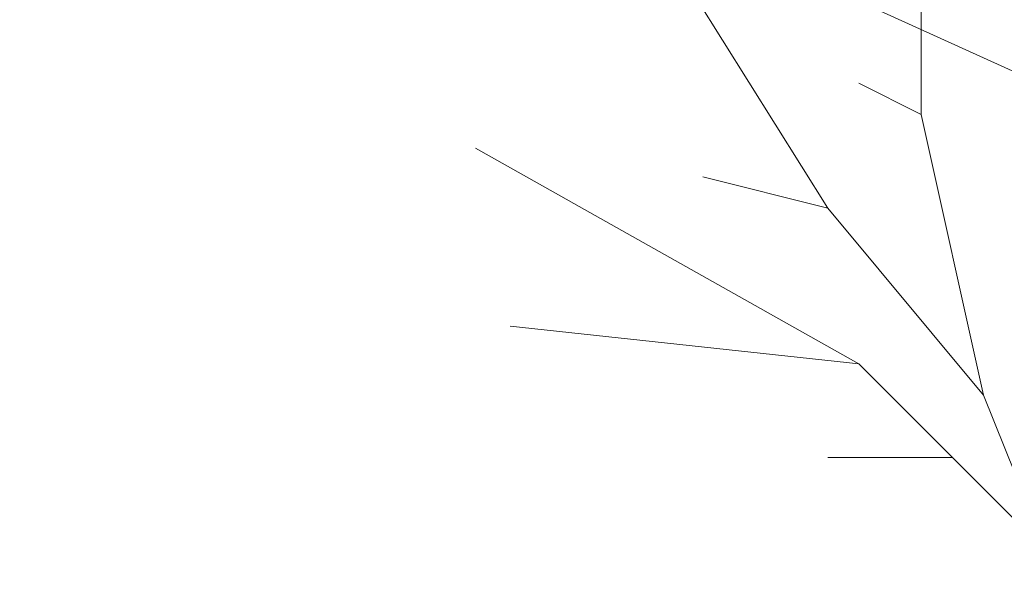
# Model space of a CAD drawing. Units: inches. Extents: x 2091 to 2899, y 967 to 2217.
# Tile 104 of 256: x 2238.36 to 2253.52, y 1105.17 to 1113.86. Entities that reach past the tile are written whole.
import ezdxf

# ---------------------------------------------------------------- set-up
doc = ezdxf.new("R2010")
doc.units = ezdxf.units.IN
doc.layers.add('A-ANNO-DIMS', color=2, linetype='Continuous', lineweight=18)
doc.layers.add('L-PLNT-TREE', color=94, linetype='Continuous', lineweight=13)
doc.layers.add('A-WALL-PATT', color=141, linetype='Continuous', lineweight=13, true_color=0xadddf7)
doc.styles.get("Standard").update_dxf_attribs({"font": 'arial.ttf'})
doc.dimstyles.new('ISO-25', dxfattribs={"dimtxt": 4, "dimasz": 4, "dimexe": 1.25, "dimexo": 0.625, "dimtad": 1, "dimdec": 0, "dimlunit": 3, "dimtxsty": 'Standard', "dimcen": 2.5, "dimadec": 0, "dimazin": 0, "dimtfac": 1, "dimtdec": 0, "dimtmove": 0, "dimatfit": 3, "dimfxl": 1, "dimarcsym": 0})

# ---------------------------------------------------------------- blocks, each defined once
blk = doc.blocks.new('*U29')
for p, q in [((-463.296, 280.416), (-552.577, 423.037)), ((-426.72, 316.992), (-426.72, 414.528)), ((-353.568, 316.992), (-487.68, 377.952)), ((-426.72, 316.992), (-451.104, 329.184)), ((-402.336, 207.264), (-426.72, 316.992)), ((-451.104, 219.456), (-601.0402, 303.8094)), ((-463.296, 280.416), (-512.064, 292.608)), ((-402.336, 207.264), (-463.296, 280.416)), ((-451.104, 219.456), (-587.4512, 234.2388)), ((-377.952, 146.304), (-451.104, 219.456)), ((-377.952, 146.304), (-402.336, 207.264)), ((-414.528, 182.88), (-463.296, 182.88))]:
    blk.add_line(p, q)
blk = doc.blocks.new('*D71')
at = {"layer": 'A-ANNO-DIMS', "color": 0, "lineweight": -2, "transparency": 16777216}
for p, q in [((2212.144, 1351.294), (2212.144, 969.464)), ((2452.144, 1351.294), (2452.144, 969.464)), ((2216.144, 970.714), (2448.144, 970.714))]:
    blk.add_line(p, q, dxfattribs=at)
at = {"layer": 'A-ANNO-DIMS', "color": 0, "transparency": 16777216}
for points in [[(2216.144, 971.381), (2216.144, 970.048), (2212.144, 970.714)], [(2448.144, 971.381), (2448.144, 970.048), (2452.144, 970.714)]]:
    blk.add_solid(points, dxfattribs=at)
at = {"layer": 'Defpoints', "color": 0, "transparency": 16777216}
for p in [(2212.144, 1351.919), (2452.144, 1351.919), (2452.144, 970.714)]:
    blk.add_point(p, dxfattribs=at)
at = {"layer": 'A-ANNO-DIMS', "color": 0, "transparency": 16777216, "insert": (2332.144, 973.382), "char_height": 4, "attachment_point": 5}
blk.add_mtext('20\'-0"', dxfattribs=at)
blk = doc.blocks.new('*D75')
at = {"layer": 'A-ANNO-DIMS', "color": 0, "lineweight": -2, "transparency": 16777216}
for p, q in [((2212.144, 1274.794), (2212.144, 969.464)), ((2308.144, 1274.794), (2308.144, 969.464)), ((2216.144, 970.714), (2304.144, 970.714))]:
    blk.add_line(p, q, dxfattribs=at)
at = {"layer": 'A-ANNO-DIMS', "color": 0, "transparency": 16777216}
for points in [[(2216.144, 971.381), (2216.144, 970.048), (2212.144, 970.714)], [(2304.144, 971.381), (2304.144, 970.048), (2308.144, 970.714)]]:
    blk.add_solid(points, dxfattribs=at)
at = {"layer": 'Defpoints', "color": 0, "transparency": 16777216}
for p in [(2212.144, 1275.419), (2308.144, 1275.419), (2308.144, 970.714)]:
    blk.add_point(p, dxfattribs=at)
at = {"layer": 'A-ANNO-DIMS', "color": 0, "transparency": 16777216, "insert": (2260.144, 973.382), "char_height": 4, "attachment_point": 5}
blk.add_mtext('8\'-0"', dxfattribs=at)

msp = doc.modelspace()

# ---------------------------------------------------------------- hatches: boundary and pattern name
at = {"layer": 'A-WALL-PATT'}
h = msp.add_hatch(color=256, dxfattribs=at)
h.dxf.hatch_style = 1
h.paths.add_polyline_path([(2803.144, 2050.919), (2203.144, 2050.919), (2203.144, 1090.919), (2803.144, 1090.919)])
h.paths.add_polyline_path([(2635.799, 1147.54), (2674.524, 1147.54, 0.376086), (2678.53, 1152.88), (2678.53, 1159.556, 0.333335), (2674.524, 1163.562), (2674.524, 1163.562), (2674.524, 1192.934), (2635.806, 1192.934), (2597.088, 1192.934), (2597.088, 1163.562, 0.333335), (2593.082, 1159.556), (2593.082, 1152.88, 0.376086), (2597.088, 1147.54)], flags=0)
h.paths.add_polyline_path([(2436.01, 1278.241, 0.000483), (2435.953, 1278.215, -0.001328), (2435.936, 1278.112, -0.001711), (2436.116, 1278.041, 0.002185)], flags=0)
h.paths.add_polyline_path([(2794.144, 1143.419), (2794.144, 1347.419), (2543.37, 1347.419), (2543.37, 1351.919), (2794.144, 1351.919), (2794.144, 1392.714), (2793.947, 1392.714), (2793.947, 1473.537), (2794.144, 1473.537), (2794.144, 1531.919), (2650.144, 1531.919), (2650.144, 1536.419), (2794.144, 1536.419), (2794.144, 1692.419), (2609.376, 1692.419), (2609.376, 1644.419), (2604.876, 1644.419), (2604.876, 1744.919), (2609.376, 1744.919), (2609.376, 1696.919), (2794.144, 1696.919), (2794.144, 1780.919), (2609.644, 1780.919), (2493.876, 1780.919), (2493.876, 1785.419), (2609.644, 1785.419), (2794.144, 1785.419), (2794.144, 1847.939), (2793.951, 1847.939), (2793.951, 1928.762), (2794.144, 1928.762), (2794.144, 1941.419), (2614.144, 1941.419), (2614.144, 1821.419), (2609.644, 1821.419), (2609.644, 1941.419), (2392.144, 1941.419), (2392.144, 1819.919), (2387.644, 1819.919), (2387.644, 1941.419), (2212.144, 1941.419), (2212.144, 1783.919), (2392.144, 1783.919), (2392.144, 1780.919), (2212.144, 1780.919), (2212.144, 1629.419), (2387.644, 1629.419), (2387.644, 1744.919), (2392.144, 1744.919), (2392.144, 1627.919), (2317.144, 1627.919), (2317.144, 1551.419), (2317.144, 1536.419), (2459.384, 1536.419), (2459.384, 1602.396), (2463.884, 1602.396), (2463.884, 1531.919), (2456.644, 1531.919), (2456.644, 1529.919), (2452.144, 1529.919), (2452.144, 1531.919), (2312.644, 1531.919), (2312.644, 1551.419), (2306.144, 1551.419), (2306.144, 1555.919), (2308.144, 1555.919), (2308.144, 1551.419), (2312.644, 1551.419), (2312.644, 1627.919), (2212.144, 1627.919), (2212.144, 1555.919), (2270.144, 1555.919), (2270.144, 1551.419), (2212.144, 1551.419), (2212.144, 1351.919), (2272.144, 1351.919), (2272.144, 1347.419), (2212.144, 1347.419), (2212.144, 1275.419), (2308.144, 1275.419), (2308.144, 1351.919), (2452.144, 1351.919), (2452.144, 1493.919), (2456.644, 1493.919), (2456.644, 1347.419), (2312.644, 1347.419), (2312.644, 1270.919), (2212.144, 1270.919), (2212.144, 1099.919), (2281.238, 1099.919), (2282.871, 1110.914), (2282.008, 1116.997), (2278.558, 1121.42), (2268.206, 1128.056), (2272.088, 1128.056), (2273.813, 1131.927), (2279.42, 1134.692), (2285.028, 1135.245), (2287.616, 1137.457), (2288.047, 1138.01), (2289.341, 1140.775), (2291.067, 1139.669), (2292.361, 1135.245), (2295.38, 1136.904), (2296.243, 1135.798), (2297.105, 1133.033), (2300.125, 1138.01), (2303.144, 1138.01), (2304.438, 1135.798), (2303.144, 1133.586), (2306.595, 1134.692), (2307.889, 1133.033), (2310.908, 1135.245), (2313.927, 1134.139), (2315.627, 1132.427), (2308.32, 1117.55), (2290.204, 1109.808), (2288.91, 1103.172), (2289.272, 1099.919), (2434.918, 1099.919), (2431.593, 1124.788), (2429.93, 1169.553), (2430.927, 1240.52), (2435.659, 1238.186), (2437.135, 1196.554), (2438.798, 1143.973), (2442.678, 1111.998), (2446.558, 1099.919), (2794.144, 1099.919), (2794.144, 1138.919), (2548.032, 1138.919), (2548.032, 1143.419), (2548.032, 1148.819), (2546.668, 1148.032), (2528.686, 1179.179, 0.256256), (2512.032, 1148.819), (2512.032, 1143.419), (2512.032, 1138.919), (2507.532, 1138.919), (2507.532, 1143.419), (2507.532, 1148.819, 0.256256), (2490.879, 1179.179), (2472.896, 1148.032), (2471.532, 1148.819), (2471.532, 1143.419), (2467.032, 1143.419), (2467.032, 1269.946, 0.039061), (2460.91, 1273.58), (2467.032, 1273.58), (2467.032, 1286.325, 0.014511), (2465.216, 1286.762), (2467.032, 1287.053), (2467.032, 1323.419), (2471.532, 1323.419), (2471.532, 1148.819), (2489.532, 1179.996), (2490.896, 1179.208), (2490.879, 1179.179, -0.256256), (2507.532, 1148.819), (2507.532, 1143.419), (2512.032, 1143.419), (2512.032, 1148.819, -0.256256), (2528.686, 1179.179), (2528.668, 1179.208), (2530.032, 1179.996), (2548.032, 1148.819), (2548.032, 1143.419)], flags=16)
h.paths.add_polyline_path([(2607.769, 1200.945), (2607.769, 1265.031), (2597.088, 1281.052), (2619.785, 1281.052), (2627.795, 1337.127), (2635.799, 1337.127), (2643.817, 1337.127), (2651.827, 1281.052), (2674.524, 1281.052), (2663.843, 1265.031), (2663.843, 1200.945), (2635.806, 1200.945)], flags=0)
edge = h.paths.add_edge_path(flags=0)
edge.add_ellipse((13303.896, 1272.999), major_axis=(-10595.313, 0), ratio=0.84230387, start_angle=0.6282372, end_angle=0.6465541, ccw=False)
edge.add_ellipse((2711.7, 1156.853), major_axis=(2.22, 0), ratio=0.842304, start_angle=111.5352, end_angle=180.6282, ccw=False)
edge.add_ellipse((13303.156, 1272.999), major_axis=(-10593.026, 0), ratio=0.84230387, start_angle=0.5282715, end_angle=0.6465541, ccw=False)
edge.add_line((2710.765, 1175.333), (2710.13, 1175.333))
edge.add_ellipse((2710.13, 1176.58), major_axis=(1.48, 0), ratio=0.842304, start_angle=180, end_angle=270, ccw=False)
edge.add_line((2708.65, 1176.58), (2708.65, 1200.783))
edge.add_ellipse((2710.13, 1200.783), major_axis=(1.48, 0), ratio=0.842304, start_angle=90, end_angle=180, ccw=False)
edge.add_line((2710.13, 1202.029), (2710.465, 1202.029))
edge.add_ellipse((13303.156, 1272.999), major_axis=(-10593.026, 0), ratio=0.84230387, start_angle=-0.0902291, end_angle=0.3838668, ccw=False)
edge.add_ellipse((2710.13, 1290.927), major_axis=(-1.48, 0), ratio=0.842304, start_angle=0, end_angle=90, ccw=False)
edge.add_line((2708.65, 1290.927), (2708.65, 1315.13))
edge.add_ellipse((2710.13, 1315.13), major_axis=(-1.48, 0), ratio=0.842304, start_angle=-90, end_angle=0, ccw=False)
edge.add_line((2710.13, 1316.377), (2710.706, 1316.377))
edge.add_ellipse((3238.402, 1296.29), major_axis=(528.234, 0), ratio=0.8423039, start_angle=176.34957, end_angle=177.82005, ccw=False)
edge.add_ellipse((2775.063, 1071.451), major_axis=(313.308, 0), ratio=0.8423039, start_angle=102.12597, end_angle=103.78053, ccw=False)
edge.add_ellipse((2775.063, 1078.306), major_axis=(-305.303, 0), ratio=0.8423039, start_angle=-79.79046, end_angle=-77.55537, ccw=False)
edge.add_ellipse((2695.142, 1541.975), major_axis=(-250.96, 0), ratio=0.8423039, start_angle=99.25657, end_angle=102.55493)
edge.add_line((2741.41, 1334.214), (2747.133, 1337.378))
edge.add_ellipse((2747.539, 1336.857), major_axis=(-0.74, 0), ratio=0.842304, start_angle=270, end_angle=307.9331, ccw=False)
edge.add_ellipse((2747.539, 1336.857), major_axis=(-0.74, 0), ratio=0.842304, start_angle=232.0669, end_angle=270, ccw=False)
edge.add_line((2747.945, 1337.378), (2753.667, 1334.214))
edge.add_ellipse((2799.935, 1541.975), major_axis=(250.96, 0), ratio=0.8423039, start_angle=257.44507, end_angle=260.74343)
edge.add_ellipse((2720.014, 1078.306), major_axis=(305.303, 0), ratio=0.8423039, start_angle=77.55537, end_angle=79.79046, ccw=False)
edge.add_ellipse((2720.014, 1071.451), major_axis=(-313.308, 0), ratio=0.8423039, start_angle=256.21947, end_angle=257.87403, ccw=False)
edge.add_ellipse((2256.676, 1296.29), major_axis=(-528.234, 0), ratio=0.8423039, start_angle=182.17995, end_angle=183.65043, ccw=False)
edge.add_line((2784.371, 1316.377), (2784.947, 1316.377))
edge.add_ellipse((2784.947, 1315.13), major_axis=(1.48, 0), ratio=0.842304, start_angle=0, end_angle=90, ccw=False)
edge.add_line((2786.427, 1315.13), (2786.427, 1290.927))
edge.add_ellipse((2784.947, 1290.927), major_axis=(1.48, 0), ratio=0.842304, start_angle=270, end_angle=360, ccw=False)
edge.add_ellipse((-7808.079, 1272.999), major_axis=(10593.026, 0), ratio=0.84230387, start_angle=-0.3838668, end_angle=0.0902291, ccw=False)
edge.add_line((2784.612, 1202.029), (2784.947, 1202.029))
edge.add_ellipse((2784.947, 1200.783), major_axis=(1.48, 0), ratio=0.842304, start_angle=0, end_angle=90, ccw=False)
edge.add_line((2786.427, 1200.783), (2786.427, 1176.58))
edge.add_ellipse((2784.947, 1176.58), major_axis=(-1.48, 0), ratio=0.842304, start_angle=90, end_angle=180, ccw=False)
edge.add_line((2784.947, 1175.333), (2784.313, 1175.333))
edge.add_ellipse((-7808.079, 1272.999), major_axis=(10593.026, 0), ratio=0.84230387, start_angle=-0.6186432, end_angle=-0.5282715, ccw=False)
edge.add_ellipse((2783.377, 1156.853), major_axis=(-2.22, 0), ratio=0.842304, start_angle=179.3718, end_angle=248.4648, ccw=False)
edge.add_ellipse((-7808.819, 1272.999), major_axis=(-10595.313, 0), ratio=0.842303866, start_angle=179.3534459, end_angle=179.3717628, ccw=False)
edge.add_ellipse((2780.297, 1153.501), major_axis=(-5.246, 0), ratio=0.842304, start_angle=90, end_angle=179.3534, ccw=False)
edge.add_line((2780.297, 1149.082), (2714.78, 1149.082))
edge.add_ellipse((2714.78, 1153.501), major_axis=(5.246, 0), ratio=0.842304, start_angle=180.6466, end_angle=270, ccw=False)
edge = h.paths.add_edge_path(flags=0)
edge.add_line((2718.187, 1151.008), (2718.187, 1170.472))
edge.add_ellipse((2721.147, 1170.472), major_axis=(-2.96, 0), ratio=0.842304, start_angle=-90, end_angle=0, ccw=False)
edge.add_line((2721.147, 1172.965), (2773.93, 1172.965))
edge.add_ellipse((2773.93, 1170.472), major_axis=(-2.96, 0), ratio=0.842304, start_angle=180, end_angle=270, ccw=False)
edge.add_line((2776.89, 1170.472), (2776.89, 1151.008))
edge.add_line((2776.89, 1151.008), (2718.187, 1151.008))
edge = h.paths.add_edge_path(flags=0)
edge.add_line((2718.187, 1180.234), (2718.187, 1199.058))
edge.add_ellipse((2747.539, 1320.399), major_axis=(147.018, 0), ratio=0.8423039, start_angle=256.40187, end_angle=283.59813)
edge.add_line((2776.89, 1199.058), (2776.89, 1180.234))
edge.add_ellipse((2747.539, 1301.575), major_axis=(147.018, 0), ratio=0.8423039, start_angle=256.40187, end_angle=283.59813, ccw=False)
edge = h.paths.add_edge_path(flags=0)
edge.add_ellipse((13303.156, 1272.999), major_axis=(-10591.546, 0), ratio=0.84230387, start_angle=0.0555943, end_angle=0.3777642, ccw=False)
edge.add_line((2711.617, 1262.722), (2715.667, 1249.495))
edge.add_ellipse((6413.892, 1241.692), major_axis=(-3698.236, 0), ratio=0.84230387, start_angle=-0.120897, end_angle=0.364076)
edge.add_line((2715.761, 1218.192), (2711.934, 1203.167))
edge = h.paths.add_edge_path(flags=0)
edge.add_line((2718.187, 1251.075), (2716.002, 1267.45))
edge.add_ellipse((2742.151, 1202.19), major_axis=(81.773, 0), ratio=0.842304, start_angle=94.27742, end_angle=111.83495, ccw=False)
edge.add_line((2737.01, 1270.931), (2758.067, 1270.931))
edge.add_ellipse((2752.926, 1202.19), major_axis=(81.773, 0), ratio=0.842304, start_angle=68.16505, end_angle=85.72258, ccw=False)
edge.add_line((2779.075, 1267.45), (2776.89, 1251.075))
edge.add_ellipse((2750.338, 1187.885), major_axis=(79.58, 0), ratio=0.842304, start_angle=67.20809, end_angle=85.12993)
edge.add_line((2756.035, 1254.744), (2739.043, 1254.744))
edge.add_ellipse((2744.739, 1187.885), major_axis=(79.58, 0), ratio=0.842304, start_angle=94.87007, end_angle=112.79191)
edge = h.paths.add_edge_path(flags=0)
edge.add_line((2783.143, 1203.167), (2779.316, 1218.192))
edge.add_ellipse((-918.815, 1241.692), major_axis=(3698.236, 0), ratio=0.84230387, start_angle=-0.364076, end_angle=0.120897)
edge.add_line((2779.41, 1249.495), (2783.46, 1262.722))
edge.add_ellipse((-7808.079, 1272.999), major_axis=(-10591.546, 0), ratio=0.84230387, start_angle=179.6222358, end_angle=179.9444057, ccw=False)
edge = h.paths.add_edge_path(flags=0)
edge.add_ellipse((2734.201, 1286.69), major_axis=(-0.357, 6.34), ratio=0.603834, start_angle=89.002, end_angle=253.6574, ccw=False)
edge.add_line((2730.369, 1286.542), (2730.369, 1301.352))
edge.add_line((2730.369, 1301.352), (2735.913, 1305.215))
edge.add_ellipse((2736.385, 1304.735), major_axis=(0.74, 0), ratio=0.842304, start_angle=90, end_angle=134.4802, ccw=False)
edge.add_line((2736.385, 1305.358), (2738.033, 1305.358))
edge.add_line((2738.033, 1305.358), (2738.033, 1307.708))
edge.add_ellipse((2794.202, 1307.708), major_axis=(56.169, 0), ratio=0.842304, start_angle=150.5614, end_angle=180, ccw=False)
edge.add_ellipse((2700.876, 1307.708), major_axis=(-56.169, 0), ratio=0.842304, start_angle=180, end_angle=209.4386, ccw=False)
edge.add_line((2757.044, 1307.708), (2757.044, 1305.358))
edge.add_line((2757.044, 1305.358), (2758.692, 1305.358))
edge.add_ellipse((2758.692, 1304.735), major_axis=(-0.74, 0), ratio=0.842304, start_angle=225.5198, end_angle=270, ccw=False)
edge.add_line((2759.164, 1305.215), (2764.708, 1301.352))
edge.add_line((2764.708, 1301.352), (2764.708, 1286.542))
edge.add_ellipse((2760.876, 1286.69), major_axis=(0.357, 6.34), ratio=0.603834, start_angle=106.3426, end_angle=270.998, ccw=False)
edge.add_line((2757.044, 1285.797), (2757.044, 1307.708))
edge.add_ellipse((2700.876, 1307.708), major_axis=(-56.169, 0), ratio=0.842304, start_angle=180, end_angle=209.4386)
edge.add_ellipse((2794.202, 1307.708), major_axis=(56.169, 0), ratio=0.842304, start_angle=150.5614, end_angle=180)
edge.add_line((2738.033, 1307.708), (2738.033, 1285.797))
h.paths.add_polyline_path([(2417.812, 1104.45), (2413.492, 1102.53), (2410.612, 1103.97), (2409.172, 1106.37), (2407.252, 1107.33), (2406.292, 1109.73), (2405.332, 1114.05), (2405.332, 1117.89), (2406.292, 1120.13), (2407.252, 1119.81), (2408.848, 1118.328), (2410.174, 1119.424), (2410.211, 1120.406), (2411.041, 1121.419), (2410.699, 1119.859), (2410.174, 1119.424), (2410.088, 1117.176), (2411.133, 1116.206), (2413.972, 1119.33), (2416.852, 1120.77), (2416.87, 1120.799), (2417.035, 1119.405), (2417.896, 1118.143), (2418.292, 1118.37), (2419.544, 1120.039), (2419.361, 1118.387), (2419.032, 1119.356), (2418.399, 1118.512), (2419.252, 1114.53), (2418.794, 1107.199)], flags=0)
h.paths.add_polyline_path([(2508.87, 1347.419), (2508.37, 1347.419), (2508.37, 1351.919), (2508.87, 1351.919)], flags=0)
h.paths.add_polyline_path([(2473.37, 1347.419), (2472.37, 1347.419), (2467.87, 1347.419), (2467.87, 1455.419), (2472.37, 1455.419), (2472.37, 1352.419), (2473.37, 1352.419)], flags=0)
h.paths.add_polyline_path([(2352.106, 1217.446), (2349.226, 1218.886), (2347.786, 1221.286), (2345.866, 1222.246), (2344.906, 1224.646), (2343.946, 1228.966), (2343.946, 1232.806), (2344.906, 1235.046), (2345.866, 1234.726), (2347.462, 1233.244), (2348.788, 1234.341), (2348.825, 1235.322), (2349.655, 1236.336), (2349.313, 1234.775), (2348.788, 1234.341), (2348.702, 1232.093), (2349.747, 1231.123), (2352.586, 1234.246), (2355.466, 1235.686), (2355.484, 1235.715), (2355.649, 1234.322), (2356.51, 1233.06), (2356.906, 1233.286), (2358.158, 1234.956), (2357.975, 1233.304), (2357.646, 1234.273), (2357.013, 1233.428), (2357.866, 1229.446), (2357.408, 1222.115), (2356.426, 1219.366)], flags=0)
h.paths.add_polyline_path([(2348.297, 1112.224), (2347.014, 1112.31), (2345.53, 1114.127), (2345.732, 1115.858), (2346.812, 1116.982), (2346.812, 1114.646), (2345.867, 1114.214), (2346.88, 1114.3)], flags=0)
h.paths.add_polyline_path([(2347.014, 1110.926), (2346.272, 1110.493), (2346.61, 1111.186)], flags=0)
h.paths.add_polyline_path([(2345.867, 1118.194), (2345.53, 1117.329), (2343.708, 1118.021), (2344.383, 1118.626)], flags=0)
h.paths.add_polyline_path([(2346.677, 1109.282), (2346.07, 1108.071), (2345.867, 1110.061)], flags=0)
h.paths.add_polyline_path([(2345.057, 1119.751), (2343.64, 1119.751), (2343.978, 1121.135)], flags=0)
h.paths.add_polyline_path([(2345.26, 1116.55), (2345.125, 1115.858), (2344.922, 1115.685), (2344.72, 1116.377)], flags=0)
h.paths.add_polyline_path([(2345.665, 1112.31), (2345.462, 1111.532), (2344.045, 1111.964), (2344.652, 1112.57)], flags=0)
h.paths.add_polyline_path([(2345.192, 1113.349), (2344.45, 1113.868), (2344.72, 1114.387)], flags=0)
h.paths.add_polyline_path([(2344.652, 1116.809), (2344.18, 1115.685), (2344.652, 1115.339), (2343.91, 1114.906), (2343.033, 1115.944), (2343.64, 1116.463)], flags=0)
h.paths.add_polyline_path([(2345.867, 1106.686), (2344.99, 1105.562), (2344.517, 1106.6)], flags=0)
h.paths.add_polyline_path([(2344.855, 1110.061), (2344.517, 1109.282), (2344.113, 1109.715)], flags=0)
h.paths.add_polyline_path([(2344.045, 1113.522), (2343.438, 1113.089), (2342.763, 1113.954)], flags=0)
h.paths.add_polyline_path([(2344.315, 1111.012), (2342.965, 1110.32), (2342.965, 1111.099)], flags=0)
h.paths.add_polyline_path([(2345.125, 1104.697), (2344.585, 1103.745), (2344.45, 1104.264)], flags=0)
h.paths.add_polyline_path([(2342.83, 1121.222), (2341.75, 1120.53), (2340.536, 1121.049), (2340.131, 1121.828), (2340.671, 1122.952), (2341.143, 1121.828), (2341.615, 1122.001)], flags=0)
h.paths.add_polyline_path([(2342.965, 1119.751), (2343.033, 1118.453), (2342.088, 1118.021), (2342.02, 1119.491)], flags=0)
h.paths.add_polyline_path([(2342.695, 1116.896), (2341.953, 1116.636), (2342.02, 1117.329)], flags=0)
h.paths.add_polyline_path([(2343.033, 1112.224), (2342.02, 1111.791), (2341.548, 1112.224), (2342.358, 1113.349)], flags=0)
h.paths.add_polyline_path([(2343.775, 1104.437), (2342.628, 1102.88), (2342.695, 1104.61), (2343.438, 1105.129)], flags=0)
h.paths.add_polyline_path([(2342.02, 1115.079), (2340.806, 1115.512), (2340.941, 1116.377)], flags=0)
h.paths.add_polyline_path([(2341.481, 1120.097), (2341.481, 1119.405), (2341.076, 1119.578), (2341.143, 1120.097)], flags=0)
h.paths.add_polyline_path([(2341.818, 1114.473), (2340.941, 1113.089), (2340.806, 1114.56)], flags=0)
h.paths.add_polyline_path([(2341.143, 1118.54), (2340.941, 1116.982), (2339.051, 1117.675), (2339.051, 1118.626)], flags=0)
h.paths.add_polyline_path([(2342.695, 1101.668), (2341.953, 1101.841), (2342.56, 1102.361)], flags=0)
h.paths.add_polyline_path([(2340.333, 1119.665), (2338.444, 1119.578), (2337.904, 1120.357), (2339.658, 1120.616)], flags=0)
h.paths.add_polyline_path([(2340.333, 1115.339), (2340.063, 1113.695), (2339.388, 1115.339)], flags=0)
h.paths.add_polyline_path([(2341.818, 1103.831), (2341.548, 1102.88), (2341.143, 1103.658)], flags=0)
h.paths.add_polyline_path([(2339.051, 1122.866), (2337.296, 1121.828), (2337.094, 1123.125), (2337.769, 1123.818)], flags=0)
h.paths.add_polyline_path([(2339.118, 1121.741), (2338.848, 1121.222), (2338.174, 1121.049), (2338.376, 1121.568)], flags=0)
h.paths.add_polyline_path([(2339.186, 1119.319), (2338.646, 1118.713), (2338.241, 1118.107), (2338.241, 1118.886)], flags=0)
h.paths.add_polyline_path([(2341.143, 1101.928), (2340.603, 1101.236), (2340.063, 1101.841), (2340.603, 1102.361)], flags=0)
h.paths.add_polyline_path([(2337.634, 1117.761), (2336.621, 1118.28), (2337.296, 1118.972)], flags=0)
h.paths.add_polyline_path([(2336.824, 1119.578), (2334.799, 1118.972), (2335.204, 1120.357), (2336.554, 1120.876)], flags=0)
h.paths.add_polyline_path([(2339.118, 1100.457), (2337.364, 1100.543), (2336.756, 1101.236)], flags=0)
h.paths.add_polyline_path([(2336.351, 1122.433), (2336.014, 1121.914), (2334.934, 1122.433), (2334.529, 1123.471), (2335.744, 1122.779)], flags=0)
h.paths.add_polyline_path([(2334.732, 1120.876), (2334.259, 1120.357), (2334.057, 1120.789), (2334.597, 1121.308)], flags=0)
h.paths.add_polyline_path([(2334.462, 1122.174), (2332.572, 1121.308), (2331.357, 1122.174), (2332.1, 1122.866)], flags=0)
h.paths.add_polyline_path([(2334.259, 1118.54), (2333.382, 1118.453), (2333.652, 1119.319)], flags=0)
h.paths.add_polyline_path([(2335.542, 1102.274), (2334.192, 1102.62), (2335.272, 1103.312)], flags=0)
h.paths.add_polyline_path([(2332.707, 1119.665), (2331.695, 1120.443), (2332.505, 1120.789)], flags=0)
h.paths.add_polyline_path([(2334.732, 1101.149), (2333.517, 1101.582), (2333.989, 1101.755)], flags=0)
h.paths.add_polyline_path([(2332.64, 1116.636), (2331.087, 1116.29), (2331.965, 1118.194)], flags=0)
h.paths.add_polyline_path([(2330.75, 1121.568), (2330.277, 1120.27), (2328.523, 1119.319), (2328.995, 1121.049)], flags=0)
h.paths.add_polyline_path([(2330.75, 1118.626), (2330.008, 1117.502), (2329.873, 1118.021)], flags=0)
h.paths.add_polyline_path([(2332.1, 1102.361), (2330.547, 1102.014), (2331.695, 1102.966)], flags=0)
h.paths.add_polyline_path([(2329.535, 1113.608), (2329.063, 1112.31), (2328.59, 1113.349)], flags=0)
h.paths.add_polyline_path([(2328.388, 1117.848), (2327.51, 1116.55), (2327.173, 1117.761)], flags=0)
h.paths.add_polyline_path([(2329.738, 1106.513), (2329.535, 1105.302), (2328.253, 1106.081)], flags=0)
h.paths.add_polyline_path([(2328.658, 1114.387), (2328.05, 1114.127), (2328.32, 1114.906)], flags=0)
h.paths.add_polyline_path([(2328.32, 1112.224), (2327.106, 1112.137), (2326.701, 1112.656)], flags=0)
h.paths.add_polyline_path([(2326.903, 1115.252), (2326.701, 1114.127), (2325.216, 1113.608), (2326.093, 1115.339)], flags=0)
h.paths.add_polyline_path([(2326.633, 1108.33), (2326.093, 1107.379), (2325.891, 1108.503), (2326.498, 1109.109)], flags=0)
h.paths.add_polyline_path([(2615.144, 1531.919), (2609.644, 1531.919), (2609.644, 1620.419), (2614.144, 1620.419), (2614.144, 1536.419), (2615.144, 1536.419)], flags=0)
h.paths.add_polyline_path([(2545.144, 1563.419), (2464.144, 1563.419), (2464.144, 1632.419), (2509.144, 1632.419), (2509.144, 1627.919), (2509.144, 1603.919), (2468.644, 1603.919), (2468.644, 1567.919), (2540.644, 1567.919), (2540.644, 1591.919), (2545.144, 1591.919)], flags=0)
h.paths.add_polyline_path([(2388.969, 1549.986), (2357.434, 1549.986), (2357.434, 1623.361), (2399.363, 1623.361), (2435.689, 1623.361), (2435.593, 1602.559), (2435.593, 1602.396), (2388.969, 1602.396)], flags=0)
h.paths.add_polyline_path([(2388.881, 1555.809), (2374.904, 1555.809), (2374.904, 1600.572), (2374.904, 1615.458), (2406.351, 1615.458), (2406.351, 1618.939), (2412.174, 1615.458), (2406.351, 1611.976), (2406.351, 1615.458), (2388.881, 1615.458)], flags=0)
h.paths.add_polyline_path([(2568.876, 1644.419), (2453.376, 1644.419), (2453.376, 1785.419), (2457.876, 1785.419), (2457.876, 1648.919), (2568.876, 1648.919)], flags=0)
h.paths.add_polyline_path([(2212.144, 1945.919), (2212.144, 2041.919), (2794.144, 2041.919), (2794.144, 1945.919)], flags=16)
h.paths.add_polyline_path([(2271.083, 1964.317), (2776.853, 1964.317), (2776.853, 2037.17), (2271.083, 2037.17)], flags=8)
h.paths.add_polyline_path([(2380.649, 1536.824), (2461.041, 1536.824), (2461.041, 1554.653), (2380.649, 1554.653)], flags=8)
h.paths.add_polyline_path([(2240.756, 1609.725), (2309.186, 1609.725), (2309.186, 1617.698), (2240.756, 1617.698)], flags=8)
h.paths.add_polyline_path([(2212.677, 1313.504), (2282.592, 1313.504), (2282.592, 1322.745), (2212.677, 1322.745)], flags=8)
h.paths.add_polyline_path([(2457.112, 1114.779), (2558.482, 1114.779), (2558.482, 1142.22), (2457.112, 1142.22)], flags=8)
h.paths.add_polyline_path([(2473.442, 1273.01), (2604.641, 1273.01), (2604.641, 1318.347), (2473.442, 1318.347)], flags=8)
h.paths.add_polyline_path([(2638.876, 1626.977), (2684.25, 1627.977), (2684.038, 1637.597), (2638.664, 1636.598)], flags=8)
h.paths.add_polyline_path([(2537.591, 1453.793), (2628.39, 1453.793), (2628.39, 1475.345), (2537.591, 1475.345)], flags=8)
h.paths.add_polyline_path([(2504.138, 1714.632), (2554.647, 1714.632), (2554.647, 1730.238), (2504.138, 1730.238)], flags=8)
h.paths.add_polyline_path([(2487.501, 1575.652), (2535.097, 1575.652), (2535.097, 1598.378), (2487.501, 1598.378)], flags=8)
h.paths.add_polyline_path([(2709.099, 1735.71), (2740.017, 1735.71), (2740.017, 1749.938), (2709.099, 1749.938)], flags=8)
h.paths.add_polyline_path([(2442.438, 1792.172), (2564.729, 1792.172), (2564.729, 1842), (2442.438, 1842)], flags=8)
h.paths.add_polyline_path([(2655.816, 1809.644), (2789.52, 1806.694), (2790.085, 1832.292), (2656.381, 1835.242)], flags=8)
h.paths.add_polyline_path([(2234.843, 1797.72), (2368.593, 1794.769), (2369.161, 1820.504), (2235.411, 1823.455)], flags=8)
h.paths.add_polyline_path([(2245.138, 1644.006), (2398.428, 1640.624), (2398.995, 1666.325), (2245.706, 1669.707)], flags=8)
h.paths.add_polyline_path([(2306.143, 1431.169), (2413.768, 1428.794), (2414.333, 1454.392), (2306.708, 1456.766)], flags=8)
h.paths.add_polyline_path([(2306.835, 1458.233), (2393.38, 1456.323), (2393.933, 1481.354), (2307.387, 1483.264)], flags=8)

# ---------------------------------------------------------------- block references
at = {"layer": 'L-PLNT-TREE', "xscale": 0.0393700787401575, "yscale": 0.0393700787401575, "zscale": 0.0393700787401575}
msp.add_blockref('*U29', (2269.041, 1099.919), dxfattribs=at)

# ---------------------------------------------------------------- dimensions: what is measured, and where the dimension line sits
at = {"layer": 'A-ANNO-DIMS'}
for base, p1, p2, picture, middle in [((2452.144, 970.714), (2212.144, 1351.919), (2452.144, 1351.919), '*D71', (2332.144, 973.382)), ((2308.144, 970.714), (2212.144, 1275.419), (2308.144, 1275.419), '*D75', (2260.144, 973.382))]:
    dim = msp.add_linear_dim(base=base, p1=p1, p2=p2, dimstyle='ISO-25', override={"dimdec": 1, "dimlfac": 1, "dimrnd": 0, "dimzin": 1, "dimdsep": 46, "dimlunit": 4, "dimfrac": 2}, dxfattribs=at)
    dim.commit()
    dim.dimension.update_dxf_attribs({"geometry": picture, "text_midpoint": middle})

doc.saveas('drawing.dxf')
